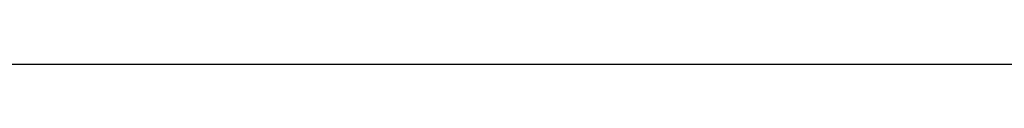
# Model space of a CAD drawing. Units: inches. Extents: x 459864 to 460310, y 324185 to 324787.
# Tile 103 of 112: x 460250.864 to 460255.113, y 324283.483 to 324283.483. Entities that reach past the tile are written whole.
import ezdxf

# ---------------------------------------------------------------- set-up
doc = ezdxf.new("R2010")
doc.units = ezdxf.units.IN
doc.layers.add('A-ANNO-DIMS', color=2, linetype='Continuous', lineweight=18)
doc.styles.get("Standard").update_dxf_attribs({"font": 'arial.ttf'})
doc.dimstyles.new('ISO-25', dxfattribs={"dimtxt": 6, "dimasz": 2.5, "dimexe": 1.25, "dimexo": 0.625, "dimtad": 1, "dimdec": 1, "dimlunit": 3, "dimtxsty": 'Standard', "dimcen": 2.5, "dimadec": 0, "dimazin": 0, "dimtfac": 1, "dimtdec": 1, "dimtmove": 0, "dimatfit": 3, "dimfxl": 1, "dimarcsym": 0})

# ---------------------------------------------------------------- blocks, each defined once
blk = doc.blocks.new('*D21')
at = {"layer": 'A-ANNO-DIMS', "color": 0, "lineweight": -2, "transparency": 16777216}
for p, q in [((460247.7399, 324715.4832), (460309.5804, 324715.4832)), ((460308.3304, 324712.9832), (460308.3304, 324285.9832)), ((460247.7399, 324283.4832), (460309.5804, 324283.4832))]:
    blk.add_line(p, q, dxfattribs=at)
at = {"layer": 'A-ANNO-DIMS', "color": 0, "transparency": 16777216}
for points in [[(460307.9137, 324712.9832), (460308.747, 324712.9832), (460308.3304, 324715.4832)], [(460307.9137, 324285.9832), (460308.747, 324285.9832), (460308.3304, 324283.4832)]]:
    blk.add_solid(points, dxfattribs=at)
at = {"layer": 'Defpoints', "color": 0, "transparency": 16777216}
for p in [(460247.1149, 324715.4832), (460247.1149, 324283.4832), (460308.3304, 324283.4832)]:
    blk.add_point(p, dxfattribs=at)
at = {"layer": 'A-ANNO-DIMS', "color": 0, "transparency": 16777216, "insert": (460304.6399, 324499.4832), "char_height": 6, "attachment_point": 5, "rotation": 90}
blk.add_mtext("36'", dxfattribs=at)
blk = doc.blocks.new('*D62')
at = {"layer": 'A-ANNO-DIMS', "color": 0, "lineweight": -2, "transparency": 16777216}
for p, q in [((460247.7399, 324332.7387), (460278.7649, 324332.7387)), ((460277.5149, 324330.2387), (460277.5149, 324285.9832)), ((460247.7399, 324283.4832), (460278.7649, 324283.4832))]:
    blk.add_line(p, q, dxfattribs=at)
at = {"layer": 'A-ANNO-DIMS', "color": 0, "transparency": 16777216}
for points in [[(460277.0983, 324330.2387), (460277.9316, 324330.2387), (460277.5149, 324332.7387)], [(460277.0983, 324285.9832), (460277.9316, 324285.9832), (460277.5149, 324283.4832)]]:
    blk.add_solid(points, dxfattribs=at)
at = {"layer": 'Defpoints', "color": 0, "transparency": 16777216}
for p in [(460247.1149, 324332.7387), (460247.1149, 324283.4832), (460277.5149, 324283.4832)]:
    blk.add_point(p, dxfattribs=at)
at = {"layer": 'A-ANNO-DIMS', "color": 0, "transparency": 16777216, "insert": (460273.7876, 324308.111), "char_height": 6, "attachment_point": 5, "rotation": 90}
blk.add_mtext('4\'-1 1/2"', dxfattribs=at)
blk = doc.blocks.new('*D65')
at = {"layer": 'A-ANNO-DIMS', "color": 0, "lineweight": -2, "transparency": 16777216}
for p, q in [((460247.7399, 324283.4832), (460302.7649, 324283.4832)), ((460301.5149, 324280.9832), (460301.5149, 324197.4832)), ((460271.7399, 324194.9832), (460302.7649, 324194.9832))]:
    blk.add_line(p, q, dxfattribs=at)
at = {"layer": 'A-ANNO-DIMS', "color": 0, "transparency": 16777216}
for points in [[(460301.0983, 324280.9832), (460301.9316, 324280.9832), (460301.5149, 324283.4832)], [(460301.0983, 324197.4832), (460301.9316, 324197.4832), (460301.5149, 324194.9832)]]:
    blk.add_solid(points, dxfattribs=at)
at = {"layer": 'Defpoints', "color": 0, "transparency": 16777216}
for p in [(460247.1149, 324283.4832), (460271.1149, 324194.9832), (460301.5149, 324194.9832)]:
    blk.add_point(p, dxfattribs=at)
at = {"layer": 'A-ANNO-DIMS', "color": 0, "transparency": 16777216, "insert": (460297.7876, 324239.2332), "char_height": 6, "attachment_point": 5, "rotation": 90}
blk.add_mtext('7\'-4 1/2"', dxfattribs=at)

msp = doc.modelspace()

# ---------------------------------------------------------------- dimensions: what is measured, and where the dimension line sits
at = {"layer": 'A-ANNO-DIMS'}
for base, p1, p2, angle, override, picture, middle in [((460308.3304, 324283.4832), (460247.1149, 324715.4832), (460247.1149, 324283.4832), 90, {"dimclrd": 0, "dimclre": 0, "dimclrt": 0}, '*D21', (460304.6399, 324499.4832)), ((460277.5149, 324283.4832), (460247.1149, 324332.7387), (460247.1149, 324283.4832), 270, {"dimdec": 1, "dimlfac": 1, "dimrnd": 0, "dimzin": 1, "dimdsep": 46, "dimlunit": 4, "dimfrac": 2}, '*D62', (460273.7876, 324308.111)), ((460301.5149, 324194.9832), (460247.1149, 324283.4832), (460271.1149, 324194.9832), 90, {"dimdec": 1, "dimlfac": 1, "dimrnd": 0, "dimzin": 1, "dimdsep": 46, "dimlunit": 4, "dimfrac": 2}, '*D65', (460297.7876, 324239.2332))]:
    dim = msp.add_linear_dim(base=base, p1=p1, p2=p2, angle=angle, dimstyle='ISO-25', override=override, dxfattribs=at)
    dim.commit()
    dim.dimension.update_dxf_attribs({"geometry": picture, "text_midpoint": middle})

doc.saveas('drawing.dxf')
